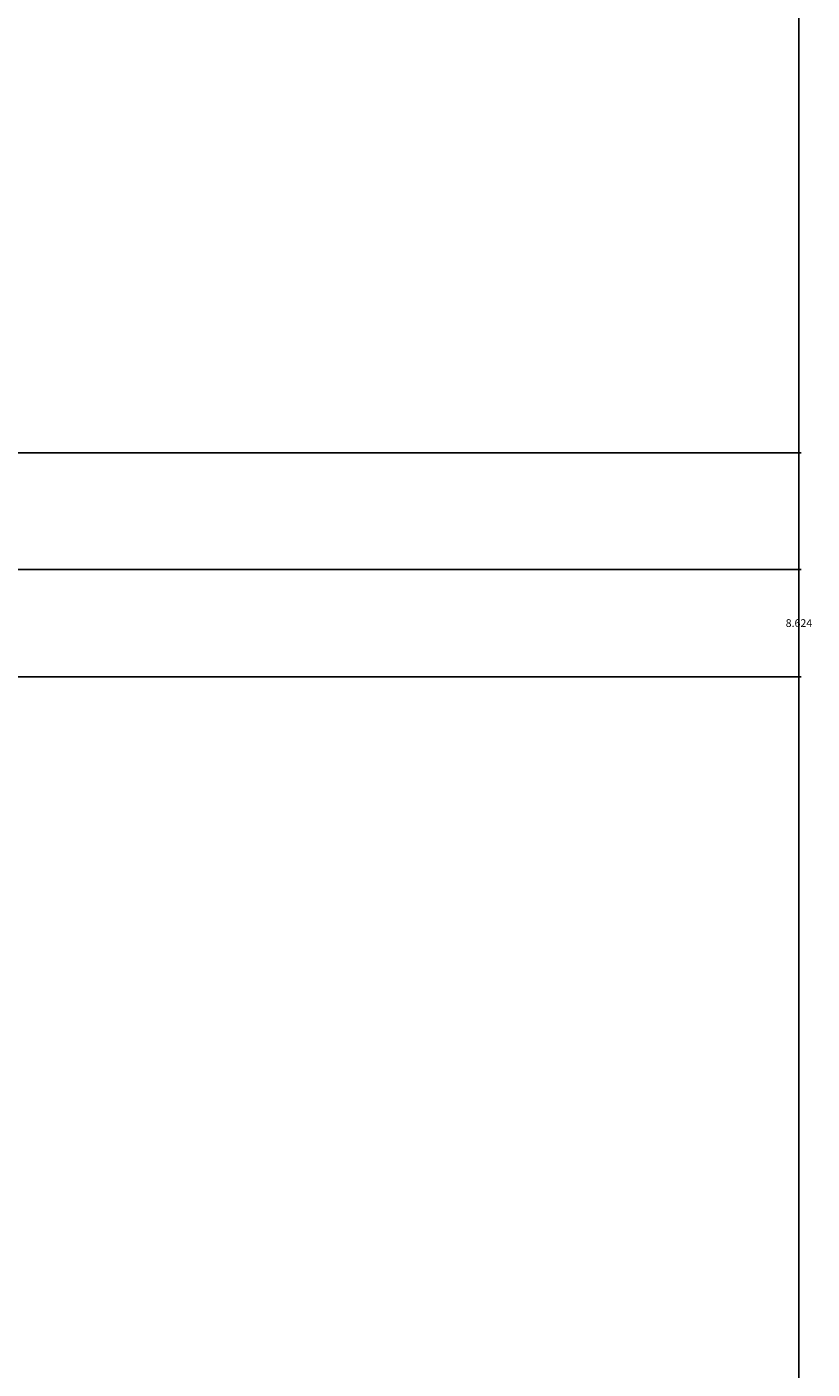
# Model space of a CAD drawing. Units: inches. Extents: x -13 to 809, y 112 to 656.
# Tile 50 of 55: x 746 to 809, y 251 to 359. Entities that reach past the tile are written whole.
import ezdxf

# ---------------------------------------------------------------- set-up
doc = ezdxf.new("R2010")
doc.units = ezdxf.units.IN
doc.header["$MEASUREMENT"] = 0
doc.layers.add('A-ANNO-DIMS', color=2, linetype='Continuous', lineweight=18)
doc.styles.get("Standard").update_dxf_attribs({"font": 'arial.ttf'})
doc.dimstyles.get("Standard").update_dxf_attribs({"dimtxt": 0.625, "dimasz": 0.18, "dimexe": 0.18, "dimexo": 0.0625, "dimgap": 0.09, "dimtad": 0, "dimtih": 1, "dimtoh": 1, "dimdec": 4, "dimzin": 0, "dimdsep": 46, "dimlunit": 4, "dimtxsty": 'Standard', "dimcen": 0.09, "dimadec": 0, "dimazin": 0, "dimtfac": 1, "dimtdec": 4, "dimtofl": 0, "dimtmove": 0, "dimatfit": 3, "dimfxl": 1, "dimtolj": 1, "dimtzin": 0, "dimarcsym": 0})

# ---------------------------------------------------------------- blocks, each defined once
blk = doc.blocks.new('*D31')
at = {"layer": 'A-ANNO-DIMS', "color": 0, "lineweight": -2, "transparency": 16777216}
for p, q in [((621.07, 617.78), (807.77, 617.78)), ((807.59, 617.6), (807.59, 384.56)), ((807.59, 150.7), (807.59, 383.74)), ((621.07, 150.52), (807.77, 150.52))]:
    blk.add_line(p, q, dxfattribs=at)
at = {"layer": 'A-ANNO-DIMS', "color": 0, "transparency": 16777216}
for points in [[(807.56, 617.6), (807.62, 617.6), (807.59, 617.78)], [(807.56, 150.7), (807.62, 150.7), (807.59, 150.52)]]:
    blk.add_solid(points, dxfattribs=at)
at = {"layer": 'Defpoints', "color": 0, "transparency": 16777216}
for p in [(621.01, 617.78), (807.59, 617.78), (621.01, 150.52)]:
    blk.add_point(p, dxfattribs=at)
at = {"layer": 'A-ANNO-DIMS', "color": 0, "transparency": 16777216, "insert": (807.59, 384.15), "char_height": 0.625, "attachment_point": 5}
blk.add_mtext('\\A1;467.3', dxfattribs=at)
blk = doc.blocks.new('*D46')
at = {"layer": 'A-ANNO-DIMS', "color": 0, "lineweight": -2, "transparency": 16777216}
for p, q in [((160.98, 408.79), (807.77, 408.79)), ((807.59, 408.61), (807.59, 367.07)), ((807.59, 324.7), (807.59, 366.25)), ((160.98, 324.52), (807.77, 324.52))]:
    blk.add_line(p, q, dxfattribs=at)
at = {"layer": 'A-ANNO-DIMS', "color": 0, "transparency": 16777216}
for points in [[(807.56, 408.61), (807.62, 408.61), (807.59, 408.79)], [(807.56, 324.7), (807.62, 324.7), (807.59, 324.52)]]:
    blk.add_solid(points, dxfattribs=at)
at = {"layer": 'Defpoints', "color": 0, "transparency": 16777216}
for p in [(160.92, 408.79), (807.59, 408.79), (160.92, 324.52)]:
    blk.add_point(p, dxfattribs=at)
at = {"layer": 'A-ANNO-DIMS', "color": 0, "transparency": 16777216, "insert": (807.59, 366.66), "char_height": 0.625, "attachment_point": 5}
blk.add_mtext('\\A1;84.27', dxfattribs=at)
blk = doc.blocks.new('*D48')
at = {"layer": 'A-ANNO-DIMS', "color": 0, "lineweight": -2, "transparency": 16777216}
for p, q in [((319.57, 444.52), (807.77, 444.52)), ((807.59, 444.34), (807.59, 384.93)), ((807.59, 324.7), (807.59, 384.11)), ((319.57, 324.52), (807.77, 324.52))]:
    blk.add_line(p, q, dxfattribs=at)
at = {"layer": 'A-ANNO-DIMS', "color": 0, "transparency": 16777216}
for points in [[(807.56, 444.34), (807.62, 444.34), (807.59, 444.52)], [(807.56, 324.7), (807.62, 324.7), (807.59, 324.52)]]:
    blk.add_solid(points, dxfattribs=at)
at = {"layer": 'Defpoints', "color": 0, "transparency": 16777216}
for p in [(319.51, 444.52), (807.59, 444.52), (319.51, 324.52)]:
    blk.add_point(p, dxfattribs=at)
at = {"layer": 'A-ANNO-DIMS', "color": 0, "transparency": 16777216, "insert": (807.59, 384.52), "char_height": 0.625, "attachment_point": 5}
blk.add_mtext('\\A1;120', dxfattribs=at)
blk = doc.blocks.new('*D106')
at = {"layer": 'A-ANNO-DIMS', "color": 0, "lineweight": -2, "transparency": 16777216}
for p, q in [((319.57, 315.14), (807.77, 315.14)), ((807.59, 314.96), (807.59, 311.24)), ((807.59, 306.7), (807.59, 310.42)), ((337.57, 306.52), (807.77, 306.52))]:
    blk.add_line(p, q, dxfattribs=at)
at = {"layer": 'A-ANNO-DIMS', "color": 0, "transparency": 16777216}
for points in [[(807.56, 314.96), (807.62, 314.96), (807.59, 315.14)], [(807.56, 306.7), (807.62, 306.7), (807.59, 306.52)]]:
    blk.add_solid(points, dxfattribs=at)
at = {"layer": 'Defpoints', "color": 0, "transparency": 16777216}
for p in [(319.51, 315.14), (807.59, 315.14), (337.51, 306.52)]:
    blk.add_point(p, dxfattribs=at)
at = {"layer": 'A-ANNO-DIMS', "color": 0, "transparency": 16777216, "insert": (807.59, 310.83), "char_height": 0.625, "attachment_point": 5}
blk.add_mtext('\\A1;8.624', dxfattribs=at)

msp = doc.modelspace()

# ---------------------------------------------------------------- dimensions: what is measured, and where the dimension line sits
at = {"layer": 'A-ANNO-DIMS'}
for base, p1, p2, override, picture, middle in [((807.5888, 617.7828), (621.008, 150.5199), (621.008, 617.7828), {"dimdec": 1, "dimlfac": 1, "dimrnd": 0, "dimzin": 0, "dimdsep": 46, "dimlunit": 2}, '*D31', (807.5888, 384.1514)), ((807.5888, 444.5199), (319.5074, 324.5199), (319.5074, 444.5199), {"dimdec": 0, "dimlfac": 1, "dimrnd": 0, "dimzin": 0, "dimdsep": 46, "dimlunit": 2}, '*D48', (807.5888, 384.5199)), ((807.5888, 408.7939), (160.9184, 324.5199), (160.9184, 408.7939), {"dimdec": 2, "dimlfac": 1, "dimrnd": 0, "dimzin": 0, "dimdsep": 46, "dimlunit": 2}, '*D46', (807.5888, 366.6569)), ((807.5888, 315.1435), (337.5074, 306.5199), (319.5074, 315.1435), {"dimdec": 3, "dimlfac": 1, "dimrnd": 0, "dimzin": 0, "dimdsep": 46, "dimlunit": 2}, '*D106', (807.5888, 310.8317))]:
    dim = msp.add_linear_dim(base=base, p1=p1, p2=p2, angle=90, dimstyle='Standard', override=override, dxfattribs=at)
    dim.commit()
    dim.dimension.update_dxf_attribs({"geometry": picture, "text_midpoint": middle})

doc.saveas('drawing.dxf')
